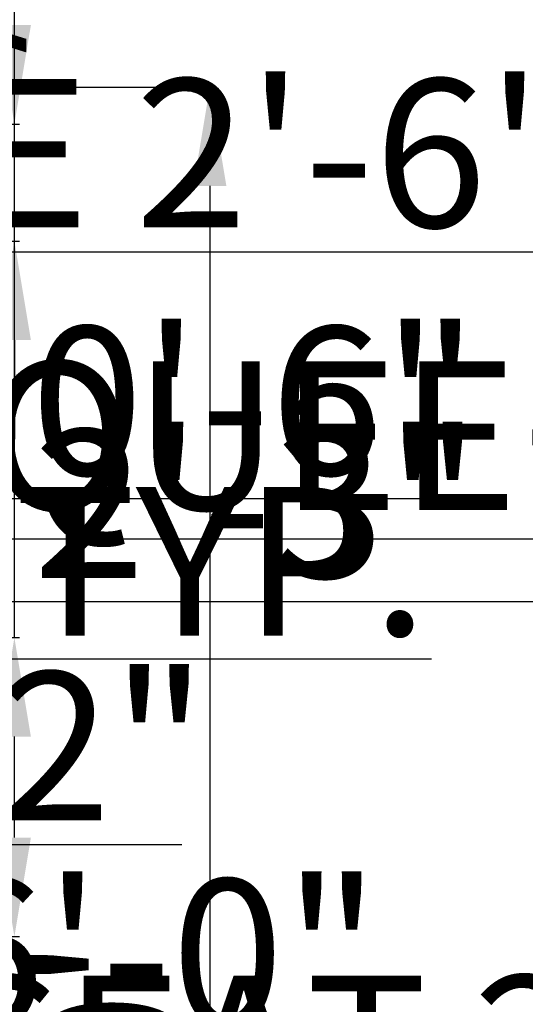
# Model space of a CAD drawing. Units: inches. Extents: x 1102 to 2414, y 295 to 1561.
# Tile 9 of 11: x 1848 to 1971, y 894 to 1133. Entities that reach past the tile are written whole.
import ezdxf

# ---------------------------------------------------------------- set-up
doc = ezdxf.new("R2010")
doc.units = ezdxf.units.IN
doc.layers.add('A-ANNO-DIMS', color=2, linetype='Continuous', lineweight=18)
doc.styles.get("Standard").update_dxf_attribs({"font": 'arial.ttf'})
doc.dimstyles.new('ISO-25', dxfattribs={"dimtxt": 36, "dimasz": 24, "dimexe": 1.25, "dimexo": 0.625, "dimtad": 1, "dimlunit": 4, "dimtxsty": 'Standard', "dimcen": 2.5, "dimadec": 0, "dimazin": 0, "dimtfac": 1, "dimtmove": 0, "dimatfit": 3, "dimfxl": 1, "dimarcsym": 0})

# ---------------------------------------------------------------- blocks, each defined once
blk = doc.blocks.new('*D3')
at = {"layer": 'A-ANNO-DIMS', "color": 0, "lineweight": -2, "transparency": 16777216}
for p, q in [((1818.17, 1116.76), (1895.42, 1116.76)), ((1894.17, 1092.76), (1894.17, 660.76)), ((1818.17, 636.76), (1895.42, 636.76))]:
    blk.add_line(p, q, dxfattribs=at)
at = {"layer": 'A-ANNO-DIMS', "color": 0, "transparency": 16777216}
for points in [[(1890.17, 1092.76), (1898.17, 1092.76), (1894.17, 1116.76)], [(1890.17, 660.76), (1898.17, 660.76), (1894.17, 636.76)]]:
    blk.add_solid(points, dxfattribs=at)
at = {"layer": 'Defpoints', "color": 0, "transparency": 16777216}
for p in [(1817.54, 1116.76), (1817.54, 636.76), (1894.17, 636.76)]:
    blk.add_point(p, dxfattribs=at)
at = {"layer": 'A-ANNO-DIMS', "color": 0, "transparency": 16777216, "insert": (1875.16, 876.76), "char_height": 36, "attachment_point": 5, "rotation": 90}
blk.add_mtext("40'", dxfattribs=at)
blk = doc.blocks.new('*D20')
at = {"layer": 'A-ANNO-DIMS', "color": 0, "lineweight": -2, "transparency": 16777216}
for p, q in [((1808.58, 695.77), (1808.58, 1020.95)), ((1806.65, 671.77), (1809.83, 671.77)), ((1808.58, 658.48), (1808.58, 671.77)), ((1806.65, 658.48), (1809.83, 658.48)), ((1808.58, 634.48), (1808.58, 610.48))]:
    blk.add_line(p, q, dxfattribs=at)
at = {"layer": 'A-ANNO-DIMS', "color": 0, "transparency": 16777216}
for points in [[(1804.58, 695.77), (1812.58, 695.77), (1808.58, 671.77)], [(1804.58, 634.48), (1812.58, 634.48), (1808.58, 658.48)]]:
    blk.add_solid(points, dxfattribs=at)
at = {"layer": 'Defpoints', "color": 0, "transparency": 16777216}
for p in [(1806.03, 671.77), (1808.58, 671.77), (1806.03, 658.48)]:
    blk.add_point(p, dxfattribs=at)
at = {"layer": 'A-ANNO-DIMS', "color": 0, "transparency": 16777216, "insert": (1789.34, 870.36), "char_height": 36, "attachment_point": 5, "rotation": 90}
blk.add_mtext('1\'-1 1/2" TYP.', dxfattribs=at)
blk = doc.blocks.new('*D23')
at = {"layer": 'A-ANNO-DIMS', "color": 0, "lineweight": -2, "transparency": 16777216}
for p, q in [((1725.8, 1018.76), (1725.8, 1005.96)), ((1806.97, 1018.76), (1806.97, 1005.96)), ((1749.8, 1007.21), (1782.97, 1007.21)), ((1806.97, 1007.21), (2238.05, 1007.21))]:
    blk.add_line(p, q, dxfattribs=at)
at = {"layer": 'A-ANNO-DIMS', "color": 0, "transparency": 16777216}
for points in [[(1749.8, 1011.21), (1749.8, 1003.21), (1725.8, 1007.21)], [(1782.97, 1011.21), (1782.97, 1003.21), (1806.97, 1007.21)]]:
    blk.add_solid(points, dxfattribs=at)
at = {"layer": 'Defpoints', "color": 0, "transparency": 16777216}
for p in [(1725.8, 1019.39), (1806.97, 1019.39), (1806.97, 1007.21)]:
    blk.add_point(p, dxfattribs=at)
at = {"layer": 'A-ANNO-DIMS', "color": 0, "transparency": 16777216, "insert": (2034.51, 1027.55), "char_height": 36, "attachment_point": 5}
blk.add_mtext('QUEEN BED 6\'-9"', dxfattribs=at)
blk = doc.blocks.new('*D25')
at = {"layer": 'A-ANNO-DIMS', "color": 0, "lineweight": -2, "transparency": 16777216}
for p, q in [((1800.76, 877.69), (1800.76, 1221.61)), ((1796.43, 853.69), (1802.01, 853.69)), ((1800.76, 820.65), (1800.76, 853.69)), ((1796.43, 820.65), (1802.01, 820.65)), ((1800.76, 796.65), (1800.76, 772.65))]:
    blk.add_line(p, q, dxfattribs=at)
at = {"layer": 'A-ANNO-DIMS', "color": 0, "transparency": 16777216}
for points in [[(1796.76, 877.69), (1804.76, 877.69), (1800.76, 853.69)], [(1796.76, 796.65), (1804.76, 796.65), (1800.76, 820.65)]]:
    blk.add_solid(points, dxfattribs=at)
at = {"layer": 'Defpoints', "color": 0, "transparency": 16777216}
for p in [(1795.81, 853.69), (1800.76, 853.69), (1795.81, 820.65)]:
    blk.add_point(p, dxfattribs=at)
at = {"layer": 'A-ANNO-DIMS', "color": 0, "transparency": 16777216, "insert": (1781.53, 1061.65), "char_height": 36, "attachment_point": 5, "rotation": 90}
blk.add_mtext('WC 2\'-9" TYP.', dxfattribs=at)
blk = doc.blocks.new('*D28')
at = {"layer": 'A-ANNO-DIMS', "color": 0, "lineweight": -2, "transparency": 16777216}
for p, q in [((1645.54, 982.63), (1645.54, 976.83)), ((1678.54, 982.63), (1678.54, 976.83)), ((1621.54, 978.08), (1597.54, 978.08)), ((1645.54, 978.08), (1678.54, 978.08)), ((1702.54, 978.08), (1947.85, 978.08))]:
    blk.add_line(p, q, dxfattribs=at)
at = {"layer": 'A-ANNO-DIMS', "color": 0, "transparency": 16777216}
for points in [[(1621.54, 982.08), (1621.54, 974.08), (1645.54, 978.08)], [(1702.54, 982.08), (1702.54, 974.08), (1678.54, 978.08)]]:
    blk.add_solid(points, dxfattribs=at)
at = {"layer": 'Defpoints', "color": 0, "transparency": 16777216}
for p in [(1645.54, 983.26), (1678.54, 983.26), (1678.54, 978.08)]:
    blk.add_point(p, dxfattribs=at)
at = {"layer": 'A-ANNO-DIMS', "color": 0, "transparency": 16777216, "insert": (1837.19, 997.09), "char_height": 36, "attachment_point": 5}
blk.add_mtext('2\'-9" TYP.', dxfattribs=at)
blk = doc.blocks.new('*D29')
at = {"layer": 'A-ANNO-DIMS', "color": 0, "lineweight": -2, "transparency": 16777216}
for p, q in [((1806.82, 1011.76), (1806.82, 1035.76)), ((1803.17, 987.76), (1808.07, 987.76)), ((1806.82, 987.76), (1806.82, 959.26)), ((1803.17, 959.26), (1808.07, 959.26)), ((1806.82, 935.26), (1806.82, 295.33))]:
    blk.add_line(p, q, dxfattribs=at)
at = {"layer": 'A-ANNO-DIMS', "color": 0, "transparency": 16777216}
for points in [[(1802.82, 1011.76), (1810.82, 1011.76), (1806.82, 987.76)], [(1802.82, 935.26), (1810.82, 935.26), (1806.82, 959.26)]]:
    blk.add_solid(points, dxfattribs=at)
at = {"layer": 'Defpoints', "color": 0, "transparency": 16777216}
for p in [(1802.54, 987.76), (1802.54, 959.26), (1806.82, 959.26)]:
    blk.add_point(p, dxfattribs=at)
at = {"layer": 'A-ANNO-DIMS', "color": 0, "transparency": 16777216, "insert": (1787.57, 603.3), "char_height": 36, "attachment_point": 5, "rotation": 90}
blk.add_mtext('BATH DOOR 2\'-4 1/2" TYP.', dxfattribs=at)
blk = doc.blocks.new('*D30')
at = {"layer": 'A-ANNO-DIMS', "color": 0, "lineweight": -2, "transparency": 16777216}
for p, q in [((1775.54, 988.38), (1775.54, 993.28)), ((1802.54, 988.38), (1802.54, 993.28)), ((1751.54, 992.03), (1727.54, 992.03)), ((1775.54, 992.03), (1802.54, 992.03)), ((1826.54, 992.03), (2071.85, 992.03))]:
    blk.add_line(p, q, dxfattribs=at)
at = {"layer": 'A-ANNO-DIMS', "color": 0, "transparency": 16777216}
for points in [[(1751.54, 996.03), (1751.54, 988.03), (1775.54, 992.03)], [(1826.54, 996.03), (1826.54, 988.03), (1802.54, 992.03)]]:
    blk.add_solid(points, dxfattribs=at)
at = {"layer": 'Defpoints', "color": 0, "transparency": 16777216}
for p in [(1802.54, 992.03), (1775.54, 987.76), (1802.54, 987.76)]:
    blk.add_point(p, dxfattribs=at)
at = {"layer": 'A-ANNO-DIMS', "color": 0, "transparency": 16777216, "insert": (1961.19, 1011.05), "char_height": 36, "attachment_point": 5}
blk.add_mtext('2\'-3" TYP.', dxfattribs=at)
blk = doc.blocks.new('*D31')
at = {"layer": 'A-ANNO-DIMS', "color": 0, "lineweight": -2, "transparency": 16777216}
for p, q in [((1629.86, 764.63), (1629.86, 760.41)), ((1653.86, 764.63), (1653.86, 760.41)), ((1605.86, 761.66), (1581.86, 761.66)), ((1629.86, 761.66), (1653.86, 761.66)), ((1677.86, 761.66), (2225.36, 761.66))]:
    blk.add_line(p, q, dxfattribs=at)
at = {"layer": 'A-ANNO-DIMS', "color": 0, "transparency": 16777216}
for points in [[(1605.86, 765.66), (1605.86, 757.66), (1629.86, 761.66)], [(1677.86, 765.66), (1677.86, 757.66), (1653.86, 761.66)]]:
    blk.add_solid(points, dxfattribs=at)
at = {"layer": 'Defpoints', "color": 0, "transparency": 16777216}
for p in [(1629.86, 765.26), (1653.86, 765.26), (1653.86, 761.66)]:
    blk.add_point(p, dxfattribs=at)
at = {"layer": 'A-ANNO-DIMS', "color": 0, "transparency": 16777216, "insert": (1963.61, 780.91), "char_height": 36, "attachment_point": 5}
blk.add_mtext('DOOR LEAF 2\'-0" TYP.', dxfattribs=at)
blk = doc.blocks.new('*D33')
at = {"layer": 'A-ANNO-DIMS', "color": 0, "lineweight": -2, "transparency": 16777216}
for p, q in [((1623.16, 1080.7), (1623.16, 1075.57)), ((1653.16, 1080.7), (1653.16, 1075.57)), ((1599.16, 1076.82), (1575.16, 1076.82)), ((1623.16, 1076.82), (1653.16, 1076.82)), ((1677.16, 1076.82), (1989.06, 1076.82))]:
    blk.add_line(p, q, dxfattribs=at)
at = {"layer": 'A-ANNO-DIMS', "color": 0, "transparency": 16777216}
for points in [[(1599.16, 1080.82), (1599.16, 1072.82), (1623.16, 1076.82)], [(1677.16, 1080.82), (1677.16, 1072.82), (1653.16, 1076.82)]]:
    blk.add_solid(points, dxfattribs=at)
at = {"layer": 'Defpoints', "color": 0, "transparency": 16777216}
for p in [(1623.16, 1081.32), (1653.16, 1081.32), (1653.16, 1076.82)]:
    blk.add_point(p, dxfattribs=at)
at = {"layer": 'A-ANNO-DIMS', "color": 0, "transparency": 16777216, "insert": (1845.11, 1096.06), "char_height": 36, "attachment_point": 5}
blk.add_mtext('RANGE 2\'-6"', dxfattribs=at)
blk = doc.blocks.new('*D39')
at = {"layer": 'A-ANNO-DIMS', "color": 0, "lineweight": -2, "transparency": 16777216}
for p, q in [((1623.32, 855.67), (1623.32, 860.64)), ((1652.27, 855.67), (1652.27, 860.64)), ((1599.32, 859.39), (1575.32, 859.39)), ((1623.32, 859.39), (1652.27, 859.39)), ((1676.27, 859.39), (2075.12, 859.39))]:
    blk.add_line(p, q, dxfattribs=at)
at = {"layer": 'A-ANNO-DIMS', "color": 0, "transparency": 16777216}
for points in [[(1599.32, 863.39), (1599.32, 855.39), (1623.32, 859.39)], [(1676.27, 863.39), (1676.27, 855.39), (1652.27, 859.39)]]:
    blk.add_solid(points, dxfattribs=at)
at = {"layer": 'Defpoints', "color": 0, "transparency": 16777216}
for p in [(1652.27, 859.39), (1623.32, 855.05), (1652.27, 855.05)]:
    blk.add_point(p, dxfattribs=at)
at = {"layer": 'A-ANNO-DIMS', "color": 0, "transparency": 16777216, "insert": (1887.69, 878.64), "char_height": 36, "attachment_point": 5}
blk.add_mtext('LOVESEAT 2\'-5"', dxfattribs=at)
blk = doc.blocks.new('*D45')
at = {"layer": 'A-ANNO-DIMS', "color": 0, "lineweight": -2, "transparency": 16777216}
for p, q in [((1736.54, 770.38), (1736.54, 1147.26)), ((1754.54, 770.38), (1754.54, 1147.26)), ((1712.54, 1146.01), (1688.54, 1146.01)), ((1736.54, 1146.01), (1754.54, 1146.01)), ((1778.54, 1146.01), (1896.1, 1146.01))]:
    blk.add_line(p, q, dxfattribs=at)
at = {"layer": 'A-ANNO-DIMS', "color": 0, "transparency": 16777216}
for points in [[(1712.54, 1150.01), (1712.54, 1142.01), (1736.54, 1146.01)], [(1778.54, 1150.01), (1778.54, 1142.01), (1754.54, 1146.01)]]:
    blk.add_solid(points, dxfattribs=at)
at = {"layer": 'Defpoints', "color": 0, "transparency": 16777216}
for p in [(1754.54, 1146.01), (1736.54, 769.76), (1754.54, 769.76)]:
    blk.add_point(p, dxfattribs=at)
at = {"layer": 'A-ANNO-DIMS', "color": 0, "transparency": 16777216, "insert": (1849.32, 1165.02), "char_height": 36, "attachment_point": 5}
blk.add_mtext('1\'-6"', dxfattribs=at)
blk = doc.blocks.new('*D47')
at = {"layer": 'A-ANNO-DIMS', "color": 0, "lineweight": -2, "transparency": 16777216}
for p, q in [((1736.54, 854.38), (1736.54, 884.26)), ((1808.54, 854.38), (1808.54, 884.26)), ((1760.54, 883.01), (1784.54, 883.01)), ((1808.54, 883.01), (1929.69, 883.01))]:
    blk.add_line(p, q, dxfattribs=at)
at = {"layer": 'A-ANNO-DIMS', "color": 0, "transparency": 16777216}
for points in [[(1760.54, 887.01), (1760.54, 879.01), (1736.54, 883.01)], [(1784.54, 887.01), (1784.54, 879.01), (1808.54, 883.01)]]:
    blk.add_solid(points, dxfattribs=at)
at = {"layer": 'Defpoints', "color": 0, "transparency": 16777216}
for p in [(1808.54, 883.01), (1736.54, 853.76), (1808.54, 853.76)]:
    blk.add_point(p, dxfattribs=at)
at = {"layer": 'A-ANNO-DIMS', "color": 0, "transparency": 16777216, "insert": (1881.12, 902.02), "char_height": 36, "attachment_point": 5}
blk.add_mtext('6\'-0"', dxfattribs=at)
blk = doc.blocks.new('*D48')
at = {"layer": 'A-ANNO-DIMS', "color": 0, "lineweight": -2, "transparency": 16777216}
for p, q in [((1689.04, 854.38), (1689.04, 1147.26)), ((1732.04, 858.88), (1732.04, 1147.26)), ((1665.04, 1146.01), (1641.04, 1146.01)), ((1689.04, 1146.01), (1732.04, 1146.01)), ((1756.04, 1146.01), (1876.97, 1146.01))]:
    blk.add_line(p, q, dxfattribs=at)
at = {"layer": 'A-ANNO-DIMS', "color": 0, "transparency": 16777216}
for points in [[(1665.04, 1150.01), (1665.04, 1142.01), (1689.04, 1146.01)], [(1756.04, 1150.01), (1756.04, 1142.01), (1732.04, 1146.01)]]:
    blk.add_solid(points, dxfattribs=at)
at = {"layer": 'Defpoints', "color": 0, "transparency": 16777216}
for p in [(1732.04, 1146.01), (1732.04, 858.26), (1689.04, 853.76)]:
    blk.add_point(p, dxfattribs=at)
at = {"layer": 'A-ANNO-DIMS', "color": 0, "transparency": 16777216, "insert": (1828.51, 1165.03), "char_height": 36, "attachment_point": 5}
blk.add_mtext('3\'-7"', dxfattribs=at)
blk = doc.blocks.new('*D49')
at = {"layer": 'A-ANNO-DIMS', "color": 0, "lineweight": -2, "transparency": 16777216}
for p, q in [((1846.79, 983.26), (1846.79, 1188.29)), ((1809.17, 983.26), (1848.04, 983.26)), ((1846.79, 934.76), (1846.79, 959.26)), ((1809.17, 910.76), (1848.04, 910.76))]:
    blk.add_line(p, q, dxfattribs=at)
at = {"layer": 'A-ANNO-DIMS', "color": 0, "transparency": 16777216}
for points in [[(1842.79, 959.26), (1850.79, 959.26), (1846.79, 983.26)], [(1842.79, 934.76), (1850.79, 934.76), (1846.79, 910.76)]]:
    blk.add_solid(points, dxfattribs=at)
at = {"layer": 'Defpoints', "color": 0, "transparency": 16777216}
for p in [(1808.54, 983.26), (1846.79, 983.26), (1808.54, 910.76)]:
    blk.add_point(p, dxfattribs=at)
at = {"layer": 'A-ANNO-DIMS', "color": 0, "transparency": 16777216, "insert": (1827.56, 1097.77), "char_height": 36, "attachment_point": 5, "rotation": 90}
blk.add_mtext('6\'-0 1/2"', dxfattribs=at)
blk = doc.blocks.new('*D52')
at = {"layer": 'A-ANNO-DIMS', "color": 0, "lineweight": -2, "transparency": 16777216}
for p, q in [((1802.54, 988.38), (1802.54, 1018.26)), ((1808.54, 988.38), (1808.54, 1018.26)), ((1778.54, 1017.01), (1754.54, 1017.01)), ((1802.54, 1017.01), (1808.54, 1017.01)), ((1832.54, 1017.01), (1953.49, 1017.01))]:
    blk.add_line(p, q, dxfattribs=at)
at = {"layer": 'A-ANNO-DIMS', "color": 0, "transparency": 16777216}
for points in [[(1778.54, 1021.01), (1778.54, 1013.01), (1802.54, 1017.01)], [(1832.54, 1021.01), (1832.54, 1013.01), (1808.54, 1017.01)]]:
    blk.add_solid(points, dxfattribs=at)
at = {"layer": 'Defpoints', "color": 0, "transparency": 16777216}
for p in [(1808.54, 1017.01), (1802.54, 987.76), (1808.54, 987.76)]:
    blk.add_point(p, dxfattribs=at)
at = {"layer": 'A-ANNO-DIMS', "color": 0, "transparency": 16777216, "insert": (1905.02, 1036.02), "char_height": 36, "attachment_point": 5}
blk.add_mtext('0\'-6"', dxfattribs=at)
blk = doc.blocks.new('*D54')
at = {"layer": 'A-ANNO-DIMS', "color": 0, "lineweight": -2, "transparency": 16777216}
for p, q in [((1846.79, 1131.76), (1846.79, 1337.21)), ((1685.17, 1107.76), (1848.04, 1107.76)), ((1846.79, 1079.39), (1846.79, 1107.76)), ((1685.17, 1079.39), (1848.04, 1079.39)), ((1846.79, 1055.39), (1846.79, 1031.39))]:
    blk.add_line(p, q, dxfattribs=at)
at = {"layer": 'A-ANNO-DIMS', "color": 0, "transparency": 16777216}
for points in [[(1842.79, 1131.76), (1850.79, 1131.76), (1846.79, 1107.76)], [(1842.79, 1055.39), (1850.79, 1055.39), (1846.79, 1079.39)]]:
    blk.add_solid(points, dxfattribs=at)
at = {"layer": 'Defpoints', "color": 0, "transparency": 16777216}
for p in [(1684.54, 1107.76), (1846.79, 1107.76), (1684.54, 1079.39)]:
    blk.add_point(p, dxfattribs=at)
at = {"layer": 'A-ANNO-DIMS', "color": 0, "transparency": 16777216, "insert": (1827.56, 1246.48), "char_height": 36, "attachment_point": 5, "rotation": 90}
blk.add_mtext('2\'-4 1/2"', dxfattribs=at)
blk = doc.blocks.new('*D58')
at = {"layer": 'A-ANNO-DIMS', "color": 0, "lineweight": -2, "transparency": 16777216}
for p, q in [((1612.78, 904.43), (1612.78, 934.3)), ((1682.5, 904.43), (1682.5, 934.3)), ((1636.78, 933.05), (1658.5, 933.05)), ((1682.5, 933.05), (1887.33, 933.05))]:
    blk.add_line(p, q, dxfattribs=at)
at = {"layer": 'A-ANNO-DIMS', "color": 0, "transparency": 16777216}
for points in [[(1636.78, 937.05), (1636.78, 929.05), (1612.78, 933.05)], [(1658.5, 937.05), (1658.5, 929.05), (1682.5, 933.05)]]:
    blk.add_solid(points, dxfattribs=at)
at = {"layer": 'Defpoints', "color": 0, "transparency": 16777216}
for p in [(1682.5, 933.05), (1612.78, 903.8), (1682.5, 903.8)]:
    blk.add_point(p, dxfattribs=at)
at = {"layer": 'A-ANNO-DIMS', "color": 0, "transparency": 16777216, "insert": (1796.92, 952.29), "char_height": 36, "attachment_point": 5}
blk.add_mtext('5\'-9 1/2"', dxfattribs=at)
blk = doc.blocks.new('*D60')
at = {"layer": 'A-ANNO-DIMS', "color": 0, "lineweight": -2, "transparency": 16777216}
for p, q in [((1586.54, 1108.38), (1586.54, 1147.26)), ((1623.16, 1107.95), (1623.16, 1147.26)), ((1562.54, 1146.01), (1538.54, 1146.01)), ((1586.54, 1146.01), (1623.16, 1146.01)), ((1647.16, 1146.01), (1851.97, 1146.01))]:
    blk.add_line(p, q, dxfattribs=at)
at = {"layer": 'A-ANNO-DIMS', "color": 0, "transparency": 16777216}
for points in [[(1562.54, 1150.01), (1562.54, 1142.01), (1586.54, 1146.01)], [(1647.16, 1150.01), (1647.16, 1142.01), (1623.16, 1146.01)]]:
    blk.add_solid(points, dxfattribs=at)
at = {"layer": 'Defpoints', "color": 0, "transparency": 16777216}
for p in [(1623.16, 1146.01), (1586.54, 1107.76), (1623.16, 1107.32)]:
    blk.add_point(p, dxfattribs=at)
at = {"layer": 'A-ANNO-DIMS', "color": 0, "transparency": 16777216, "insert": (1761.57, 1165.26), "char_height": 36, "attachment_point": 5}
blk.add_mtext('3\'-0 1/2"', dxfattribs=at)
blk = doc.blocks.new('*D62')
at = {"layer": 'A-ANNO-DIMS', "color": 0, "lineweight": -2, "transparency": 16777216}
for p, q in [((1778.54, 982.63), (1778.54, 606.26)), ((1802.54, 982.63), (1802.54, 606.26)), ((1754.54, 607.51), (1730.54, 607.51)), ((1778.54, 607.51), (1802.54, 607.51)), ((1826.54, 607.51), (1948.11, 607.51))]:
    blk.add_line(p, q, dxfattribs=at)
at = {"layer": 'A-ANNO-DIMS', "color": 0, "transparency": 16777216}
for points in [[(1754.54, 611.51), (1754.54, 603.51), (1778.54, 607.51)], [(1826.54, 611.51), (1826.54, 603.51), (1802.54, 607.51)]]:
    blk.add_solid(points, dxfattribs=at)
at = {"layer": 'Defpoints', "color": 0, "transparency": 16777216}
for p in [(1778.54, 983.26), (1802.54, 983.26), (1802.54, 607.51)]:
    blk.add_point(p, dxfattribs=at)
at = {"layer": 'A-ANNO-DIMS', "color": 0, "transparency": 16777216, "insert": (1899.32, 626.52), "char_height": 36, "attachment_point": 5}
blk.add_mtext('2\'-0"', dxfattribs=at)
blk = doc.blocks.new('*D64')
at = {"layer": 'A-ANNO-DIMS', "color": 0, "lineweight": -2, "transparency": 16777216}
for p, q in [((1695.04, 982.63), (1695.04, 606.26)), ((1719.04, 982.63), (1719.04, 606.26)), ((1671.04, 607.51), (1647.04, 607.51)), ((1695.04, 607.51), (1719.04, 607.51)), ((1743.04, 607.51), (1864.61, 607.51))]:
    blk.add_line(p, q, dxfattribs=at)
at = {"layer": 'A-ANNO-DIMS', "color": 0, "transparency": 16777216}
for points in [[(1671.04, 611.51), (1671.04, 603.51), (1695.04, 607.51)], [(1743.04, 611.51), (1743.04, 603.51), (1719.04, 607.51)]]:
    blk.add_solid(points, dxfattribs=at)
at = {"layer": 'Defpoints', "color": 0, "transparency": 16777216}
for p in [(1695.04, 983.26), (1719.04, 983.26), (1719.04, 607.51)]:
    blk.add_point(p, dxfattribs=at)
at = {"layer": 'A-ANNO-DIMS', "color": 0, "transparency": 16777216, "insert": (1815.82, 626.52), "char_height": 36, "attachment_point": 5}
blk.add_mtext('2\'-0"', dxfattribs=at)
blk = doc.blocks.new('*D65')
at = {"layer": 'A-ANNO-DIMS', "color": 0, "lineweight": -2, "transparency": 16777216}
for p, q in [((1697.64, 770.38), (1697.64, 1147.26)), ((1725.04, 770.38), (1725.04, 1147.26)), ((1673.64, 1146.01), (1649.64, 1146.01)), ((1697.64, 1146.01), (1725.04, 1146.01)), ((1749.04, 1146.01), (1954.49, 1146.01))]:
    blk.add_line(p, q, dxfattribs=at)
at = {"layer": 'A-ANNO-DIMS', "color": 0, "transparency": 16777216}
for points in [[(1673.64, 1150.01), (1673.64, 1142.01), (1697.64, 1146.01)], [(1749.04, 1150.01), (1749.04, 1142.01), (1725.04, 1146.01)]]:
    blk.add_solid(points, dxfattribs=at)
at = {"layer": 'Defpoints', "color": 0, "transparency": 16777216}
for p in [(1725.04, 1146.01), (1697.64, 769.76), (1725.04, 769.76)]:
    blk.add_point(p, dxfattribs=at)
at = {"layer": 'A-ANNO-DIMS', "color": 0, "transparency": 16777216, "insert": (1863.77, 1165.26), "char_height": 36, "attachment_point": 5}
blk.add_mtext('2\'-3 1/2"', dxfattribs=at)

msp = doc.modelspace()

# ---------------------------------------------------------------- dimensions: what is measured, and where the dimension line sits
at = {"layer": 'A-ANNO-DIMS'}
for base, p1, p2, picture, middle in [((1846.794, 1107.76), (1684.544, 1079.395), (1684.544, 1107.76), '*D54', (1827.555, 1246.483)), ((1846.794, 983.26), (1808.544, 910.76), (1808.544, 983.26), '*D49', (1827.555, 1097.774))]:
    dim = msp.add_linear_dim(base=base, p1=p1, p2=p2, angle=90, dimstyle='ISO-25', override={"dimdec": 1, "dimlfac": 1, "dimrnd": 0, "dimzin": 1, "dimdsep": 46, "dimlunit": 4, "dimfrac": 2}, dxfattribs=at)
    dim.commit()
    dim.dimension.update_dxf_attribs({"geometry": picture, "text_midpoint": middle})
for base, p1, p2, angle, text, picture, middle in [((1800.764, 853.692), (1795.807, 820.646), (1795.807, 853.692), 90, 'WC <> TYP.', '*D25', (1781.525, 1061.653)), ((1806.819, 959.26), (1802.544, 987.76), (1802.544, 959.26), 270, 'BATH DOOR <> TYP.', '*D29', (1787.568, 603.296)), ((1808.577, 671.77), (1806.028, 658.482), (1806.028, 671.77), 90, '<> TYP.', '*D20', (1789.338, 870.362))]:
    dim = msp.add_linear_dim(base=base, p1=p1, p2=p2, angle=angle, text=text, dimstyle='ISO-25', override={"dimdec": 1, "dimlfac": 1, "dimrnd": 0, "dimzin": 1, "dimdsep": 46, "dimlunit": 4, "dimfrac": 2}, dxfattribs=at)
    dim.commit()
    dim.dimension.update_dxf_attribs({"geometry": picture, "text_midpoint": middle})
for base, p1, p2, picture, middle in [((1623.162, 1146.01), (1586.544, 1107.76), (1623.162, 1107.321), '*D60', (1761.566, 1165.261)), ((1725.044, 1146.01), (1697.644, 769.76), (1725.044, 769.76), '*D65', (1863.767, 1165.261)), ((1732.044, 1146.01), (1689.044, 853.76), (1732.044, 858.26), '*D48', (1828.505, 1165.028)), ((1754.544, 1146.01), (1736.544, 769.76), (1754.544, 769.76), '*D45', (1849.323, 1165.015)), ((1808.544, 1017.01), (1802.544, 987.76), (1808.544, 987.76), '*D52', (1905.018, 1036.015)), ((1682.499, 933.053), (1612.778, 903.803), (1682.499, 903.803), '*D58', (1796.915, 952.292)), ((1719.044, 607.51), (1695.044, 983.26), (1719.044, 983.26), '*D64', (1815.825, 626.515)), ((1802.544, 607.51), (1778.544, 983.26), (1802.544, 983.26), '*D62', (1899.325, 626.515)), ((1808.544, 883.01), (1736.544, 853.76), (1808.544, 853.76), '*D47', (1881.116, 902.015))]:
    dim = msp.add_linear_dim(base=base, p1=p1, p2=p2, dimstyle='ISO-25', override={"dimdec": 1, "dimlfac": 1, "dimrnd": 0, "dimzin": 1, "dimdsep": 46, "dimlunit": 4, "dimfrac": 2}, dxfattribs=at)
    dim.commit()
    dim.dimension.update_dxf_attribs({"geometry": picture, "text_midpoint": middle})
for base, p1, p2, text, picture, middle in [((1653.162, 1076.821), (1623.162, 1081.321), (1653.162, 1081.321), 'RANGE <>', '*D33', (1845.112, 1096.06)), ((1806.973, 1007.211), (1725.798, 1019.387), (1806.973, 1019.387), 'QUEEN BED <>', '*D23', (2034.509, 1027.555)), ((1802.544, 992.035), (1775.544, 987.76), (1802.544, 987.76), '<> TYP.', '*D30', (1961.195, 1011.053)), ((1678.544, 978.085), (1645.544, 983.26), (1678.544, 983.26), '<> TYP.', '*D28', (1837.195, 997.09)), ((1652.268, 859.388), (1623.32, 855.046), (1652.268, 855.046), 'LOVESEAT <>', '*D39', (1887.695, 878.64)), ((1653.864, 761.66), (1629.864, 765.26), (1653.864, 765.26), 'DOOR LEAF <> TYP.', '*D31', (1963.611, 780.911))]:
    dim = msp.add_linear_dim(base=base, p1=p1, p2=p2, text=text, dimstyle='ISO-25', override={"dimdec": 1, "dimlfac": 1, "dimrnd": 0, "dimzin": 1, "dimdsep": 46, "dimlunit": 4, "dimfrac": 2}, dxfattribs=at)
    dim.commit()
    dim.dimension.update_dxf_attribs({"geometry": picture, "text_midpoint": middle})
dim = msp.add_linear_dim(base=(1894.167, 636.76), p1=(1817.544, 1116.76), p2=(1817.544, 636.76), angle=90, dimstyle='ISO-25', override={"dimclrd": 0, "dimclre": 0, "dimclrt": 0}, dxfattribs=at)
dim.commit()
dim.dimension.update_dxf_attribs({"geometry": '*D3', "text_midpoint": (1894.167, 876.76), "dimtype": 160})

doc.saveas('drawing.dxf')
